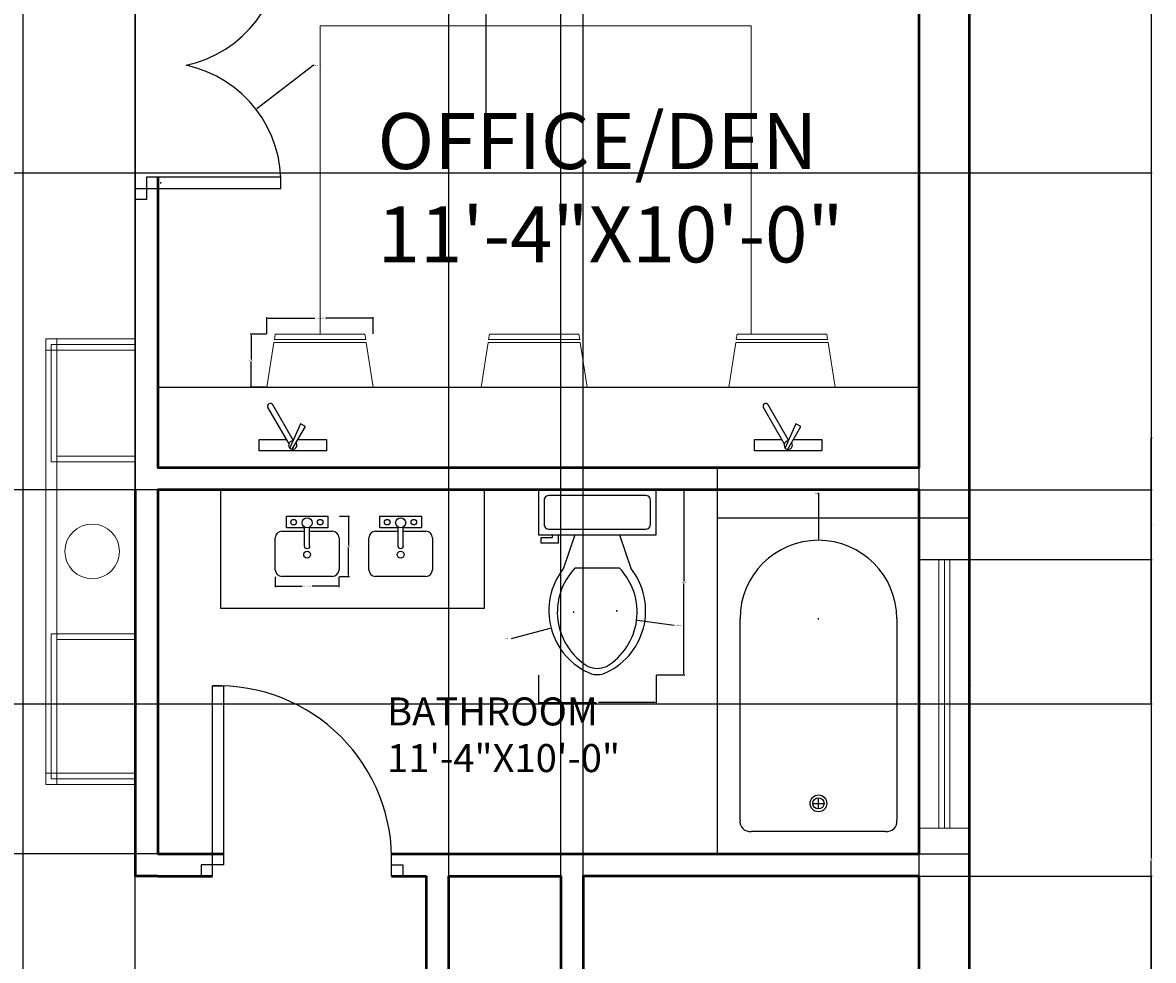
# Model space of a CAD drawing. Units: inches. Extents: x 821 to 2399, y 74 to 823.
# Tile 6 of 13: x 1128 to 1330, y 381 to 549. Entities that reach past the tile are written whole.
import ezdxf

# ---------------------------------------------------------------- set-up
doc = ezdxf.new("R2010")
doc.units = ezdxf.units.IN
doc.header["$MEASUREMENT"] = 0
doc.layers.get('0').update_dxf_attribs({"lineweight": 53})
for name, color, linetype, lineweight in [('A-ANNO-DIMS', 2, 'Continuous', 18), ('A-AREA-IDEN', 7, 'Continuous', 18), ('A-DOOR', 4, 'Continuous', 25), ('A-FLOR-CASE', 9, 'Continuous', 25), ('A-FLOR-FIXT', 8, 'Continuous', 25), ('A-FURN', 8, 'Continuous', 18), ('A-GLAZ', 4, 'Continuous', 18), ('WALLS', 7, 'Continuous', 50)]:
    doc.layers.add(name, color=color, linetype=linetype, lineweight=lineweight)
doc.styles.get("Standard").update_dxf_attribs({"font": 'arial.ttf'})
doc.dimstyles.get("Standard").update_dxf_attribs({"dimtxt": 0.18, "dimasz": 0.18, "dimexe": 0.18, "dimexo": 0.0625, "dimgap": 0.09, "dimtad": 0, "dimtih": 1, "dimtoh": 1, "dimdec": 4, "dimzin": 0, "dimdsep": 46, "dimtxsty": 'Standard', "dimcen": 0.09, "dimadec": 0, "dimazin": 0, "dimtfac": 1, "dimtdec": 4, "dimtofl": 0, "dimtmove": 0, "dimatfit": 3, "dimfxl": 1, "dimtolj": 1, "dimtzin": 0, "dimarcsym": 0})

# ---------------------------------------------------------------- blocks, each defined once
blk = doc.blocks.new('Bath Tub - 26 x 60 in.')
for p, q in [((8, -18), (10, -18)), ((9, -17), (9, -19))]:
    blk.add_line(p, q)
blk.add_lwpolyline([(0, -36), (0, 0), (60, 0), (60, -36)], close=True)
for points in [[(6, -4), (42, -4)], [(4, -30), (4, -6)], [(42, -32), (6, -32)]]:
    blk.add_lwpolyline(points)
for radius in [1.5, 1]:
    blk.add_circle((9, -18), radius)
for centre, radius, start, end in [((5.75, -5.75), 1.77, 81.8699, 188.1301), ((42, -18), 14, 270, 90), ((5.75, -30.25), 1.77, 171.8699, 278.1301)]:
    blk.add_arc(centre, radius, start, end)
blk = doc.blocks.new('Toilet - top')
for p, q in [((9.5, -6), (9.5, -2)), ((-8, -8.5), (-8, -8)), ((-7, -8), (-7, -9.5)), ((-4, -8), (-6, -14)), ((4, -8), (6, -14)), ((-10, -8.5), (-8, -8.5)), ((-10, -9.5), (-10, -8.5)), ((-7, -9.5), (-10, -9.5)), ((4, -14), (-4, -14))]:
    blk.add_line(p, q)
blk.add_lwpolyline([(10.5, -8), (10.5, 0), (-10.5, 0), (-10.5, -8)], close=True)
for points in [[(-9.5, -2), (-9.5, -6)], [(8.5, -1), (-8.5, -1)], [(-8.5, -7), (8.5, -7)]]:
    blk.add_lwpolyline(points)
for centre, radius, start, end in [((-8.62, -1.88), 0.884, 81.8699, 188.1301), ((8.62, -1.88), 0.884, 351.8699, 98.1301), ((-8.62, -6.12), 0.884, 171.8699, 278.1301), ((8.62, -6.12), 0.884, 261.8699, 8.1301), ((3.52, -21.58), 12.17, 141.4691, 247.9714), ((4.2, -21.82), 11.33, 136.3677, 238.9468), ((-3.52, -21.58), 12.17, 292.0284, 38.5307), ((-4.2, -21.82), 11.33, 301.053, 43.6321), ((0, -27.88), 4, 245.7318, 294.2682), ((0, -29), 4, 254.8605, 285.1395)]:
    blk.add_arc(centre, radius, start, end)
blk = doc.blocks.new('Faucet - single handle top')
for p, q in [((0.08, -0.26), (-2.26, -4.34)), ((-1.37, -4.79), (0.55, -0.5)), ((-0.06, -1.9), (3.57, -8.18)), ((4.43, -7.68), (0.72, -1.24)), ((-2.26, -4.34), (-1.37, -4.79))]:
    blk.add_line(p, q)
for points in [[(-0.92, -2), (-6, -2), (-6, 0), (6, 0), (6, -2), (1.16, -2)], [(-0.01, -2), (-0.12, -2)]]:
    blk.add_lwpolyline(points)
for centre, radius, start, end in [((0, -1), 0.75, 269.2246, 216.2304), ((4, -7.93), 0.5, 210, 30)]:
    blk.add_arc(centre, radius, start, end)
blk = doc.blocks.new('DOOR-SWING-32IN')
for p, q in [((0, 0), (2, 0)), ((34, 0), (36, 0))]:
    blk.add_line(p, q)
blk.add_lwpolyline([(34, 2, 0.433232), (2, 34), (4, 34), (4, 2), (2, 2), (2, 34)], format="xyb")
for points in [[(0, 0), (2, 0), (2, 2), (0, 2)], [(36, 0), (34, 0), (34, 2), (36, 2)]]:
    blk.add_lwpolyline(points, close=True)
blk = doc.blocks.new('WIN-48IN')
for p, q in [((3.5, 48), (3.5, 0)), ((4.5, 48), (4.5, 0)), ((5.5, 48), (5.5, 0))]:
    blk.add_line(p, q)
blk.add_lwpolyline([(9, 0), (0, 0), (0, 48), (9, 48)], close=True)
blk = doc.blocks.new('CHAIR-DESK-19IN')
for p, q in [((1.33, 8.5), (17.64, 8.5)), ((0, 0), (1.25, 8)), ((17.72, 8), (1.25, 8)), ((17.72, 8), (18.97, 0))]:
    blk.add_line(p, q)
blk.add_lwpolyline([(1.33, 8.5), (1.48, 9.5), (17.48, 9.5), (17.64, 8.5)])
blk = doc.blocks.new('LAV-RECT-WITH-FAUCET')
blk.add_line((6.15, 5.4), (6.15, 8.82))
for points in [[(5.25, 8.7), (2, 8.7), (2, 10.75), (5.8, 10.75)], [(5.8, 10.75), (9.4, 10.75), (9.4, 8.7), (6.15, 8.7)], [(1.2, 8.1), (5.25, 8.1)], [(6.15, 8.1), (10.2, 8.1)], [(0, 1.2), (0, 6.9)], [(11.4, 6.9), (11.4, 1.2)], [(10.2, 0), (1.2, 0)]]:
    blk.add_lwpolyline(points)
blk.add_lwpolyline([(6.15, 5.4, -1), (5.25, 5.4), (5.25, 8.82)], format="xyb")
for centre, radius in [((3.3, 9.7), 0.5), ((5.7, 9.6), 0.9), ((8.05, 9.7), 0.5), ((5.7, 3.9), 0.6)]:
    blk.add_circle(centre, radius)
for centre, start, end in [((1.28, 6.83), 93.3665, 176.6335), ((10.13, 6.83), 3.3665, 86.6335), ((1.28, 1.28), 183.3665, 266.6335), ((10.13, 1.28), 273.3665, 356.6335)]:
    blk.add_arc(centre, 1.28, start, end)
blk = doc.blocks.new('*D38')
at = {"layer": 'A-ANNO-DIMS', "color": 0, "lineweight": -2, "transparency": 16777216}
for p, q in [((1171.89, 493.43), (1171.89, 496.4)), ((1172.07, 496.22), (1180.42, 496.22)), ((1190.68, 496.22), (1182.32, 496.22)), ((1190.86, 493.43), (1190.86, 496.4))]:
    blk.add_line(p, q, dxfattribs=at)
at = {"layer": 'A-ANNO-DIMS', "color": 0, "lineweight": 50, "transparency": 16777216}
for points in [[(1172.07, 496.25), (1172.07, 496.19), (1171.89, 496.22)], [(1190.68, 496.25), (1190.68, 496.19), (1190.86, 496.22)]]:
    blk.add_solid(points, dxfattribs=at)
at = {"layer": 'Defpoints', "color": 0, "lineweight": 50, "transparency": 16777216}
for p in [(1190.86, 496.22), (1171.89, 493.37), (1190.86, 493.37)]:
    blk.add_point(p, dxfattribs=at)
at = {"layer": 'A-ANNO-DIMS', "color": 0, "transparency": 16777216, "insert": (1181.37, 496.22), "char_height": 0.18, "attachment_point": 5}
blk.add_mtext('\\A1;CHAIR 19 TYP.', dxfattribs=at)
blk = doc.blocks.new('*D39')
at = {"layer": 'A-ANNO-DIMS', "color": 0, "lineweight": -2, "transparency": 16777216}
for p, q in [((1171.82, 493.37), (1168.86, 493.37)), ((1169.04, 493.19), (1169.04, 488.8)), ((1169.04, 484.05), (1169.04, 488.44)), ((1171.82, 483.87), (1168.86, 483.87))]:
    blk.add_line(p, q, dxfattribs=at)
at = {"layer": 'A-ANNO-DIMS', "color": 0, "lineweight": 50, "transparency": 16777216}
for points in [[(1169.01, 493.19), (1169.07, 493.19), (1169.04, 493.37)], [(1169.01, 484.05), (1169.07, 484.05), (1169.04, 483.87)]]:
    blk.add_solid(points, dxfattribs=at)
at = {"layer": 'Defpoints', "color": 0, "lineweight": 50, "transparency": 16777216}
for p in [(1169.04, 493.37), (1171.89, 493.37), (1171.89, 483.87)]:
    blk.add_point(p, dxfattribs=at)
at = {"layer": 'A-ANNO-DIMS', "color": 0, "transparency": 16777216, "insert": (1169.04, 488.62), "char_height": 0.18, "attachment_point": 5}
blk.add_mtext('\\A1;10 TYP.', dxfattribs=at)
blk = doc.blocks.new('*D42')
at = {"layer": 'A-ANNO-DIMS', "color": 0, "lineweight": -2, "transparency": 16777216}
for p, q in [((1173.35, 450), (1173.35, 448.17)), ((1173.53, 448.35), (1178.12, 448.35)), ((1184.57, 448.35), (1179.99, 448.35)), ((1184.75, 450), (1184.75, 448.17))]:
    blk.add_line(p, q, dxfattribs=at)
at = {"layer": 'A-ANNO-DIMS', "color": 0, "lineweight": 50, "transparency": 16777216}
for points in [[(1173.53, 448.38), (1173.53, 448.32), (1173.35, 448.35)], [(1184.57, 448.38), (1184.57, 448.32), (1184.75, 448.35)]]:
    blk.add_solid(points, dxfattribs=at)
at = {"layer": 'Defpoints', "color": 0, "lineweight": 50, "transparency": 16777216}
for p in [(1173.35, 450.06), (1184.75, 450.06), (1184.75, 448.35)]:
    blk.add_point(p, dxfattribs=at)
at = {"layer": 'A-ANNO-DIMS', "color": 0, "transparency": 16777216, "insert": (1179.05, 448.35), "char_height": 0.18, "attachment_point": 5}
blk.add_mtext('\\A1;BASIN 11 TYP.', dxfattribs=at)
blk = doc.blocks.new('*D43')
at = {"layer": 'A-ANNO-DIMS', "color": 0, "lineweight": -2, "transparency": 16777216}
for p, q in [((1184.82, 460.81), (1186.64, 460.81)), ((1186.46, 460.63), (1186.46, 455.61)), ((1186.46, 450.24), (1186.46, 455.25)), ((1184.82, 450.06), (1186.64, 450.06))]:
    blk.add_line(p, q, dxfattribs=at)
at = {"layer": 'A-ANNO-DIMS', "color": 0, "lineweight": 50, "transparency": 16777216}
for points in [[(1186.43, 460.63), (1186.49, 460.63), (1186.46, 460.81)], [(1186.43, 450.24), (1186.49, 450.24), (1186.46, 450.06)]]:
    blk.add_solid(points, dxfattribs=at)
at = {"layer": 'Defpoints', "color": 0, "lineweight": 50, "transparency": 16777216}
for p in [(1184.75, 460.81), (1186.46, 460.81), (1184.75, 450.06)]:
    blk.add_point(p, dxfattribs=at)
at = {"layer": 'A-ANNO-DIMS', "color": 0, "transparency": 16777216, "insert": (1186.46, 455.43), "char_height": 0.18, "attachment_point": 5}
blk.add_mtext('\\A1;11 TYP.', dxfattribs=at)
blk = doc.blocks.new('*D54')
at = {"layer": 'A-ANNO-DIMS', "color": 0, "lineweight": -2, "transparency": 16777216}
for p, q in [((1288.44, 460.52), (1297.55, 460.52)), ((1297.37, 460.34), (1297.37, 430.7)), ((1297.37, 400.7), (1297.37, 430.34)), ((1288.44, 400.52), (1297.55, 400.52))]:
    blk.add_line(p, q, dxfattribs=at)
at = {"layer": 'A-ANNO-DIMS', "color": 0, "lineweight": 50, "transparency": 16777216}
for points in [[(1297.34, 460.34), (1297.4, 460.34), (1297.37, 460.52)], [(1297.34, 400.7), (1297.4, 400.7), (1297.37, 400.52)]]:
    blk.add_solid(points, dxfattribs=at)
at = {"layer": 'Defpoints', "color": 0, "lineweight": 50, "transparency": 16777216}
for p in [(1288.37, 460.52), (1297.37, 460.52), (1288.37, 400.52)]:
    blk.add_point(p, dxfattribs=at)
at = {"layer": 'A-ANNO-DIMS', "color": 0, "transparency": 16777216, "insert": (1297.37, 430.52), "char_height": 0.18, "attachment_point": 5}
blk.add_mtext('\\A1;TUB 60', dxfattribs=at)
blk = doc.blocks.new('*D55')
at = {"layer": 'A-ANNO-DIMS', "color": 0, "lineweight": -2, "transparency": 16777216}
for p, q in [((1252.37, 460.58), (1252.37, 469.7)), ((1252.55, 469.52), (1270.15, 469.52)), ((1288.19, 469.52), (1270.59, 469.52)), ((1288.37, 460.58), (1288.37, 469.7))]:
    blk.add_line(p, q, dxfattribs=at)
at = {"layer": 'A-ANNO-DIMS', "color": 0, "lineweight": 50, "transparency": 16777216}
for points in [[(1252.55, 469.55), (1252.55, 469.49), (1252.37, 469.52)], [(1288.19, 469.55), (1288.19, 469.49), (1288.37, 469.52)]]:
    blk.add_solid(points, dxfattribs=at)
at = {"layer": 'Defpoints', "color": 0, "lineweight": 50, "transparency": 16777216}
for p in [(1252.37, 469.52), (1252.37, 460.52), (1288.37, 460.52)]:
    blk.add_point(p, dxfattribs=at)
at = {"layer": 'A-ANNO-DIMS', "color": 0, "transparency": 16777216, "insert": (1270.37, 469.52), "char_height": 0.18, "attachment_point": 5}
blk.add_mtext('\\A1;36', dxfattribs=at)
blk = doc.blocks.new('*D56')
at = {"layer": 'A-ANNO-DIMS', "color": 0, "lineweight": -2, "transparency": 16777216}
for p, q in [((1241.44, 465.52), (1246.51, 465.52)), ((1246.33, 465.34), (1246.33, 449.18)), ((1246.33, 432.65), (1246.33, 448.81)), ((1241.44, 432.47), (1246.51, 432.47))]:
    blk.add_line(p, q, dxfattribs=at)
at = {"layer": 'A-ANNO-DIMS', "color": 0, "lineweight": 50, "transparency": 16777216}
for points in [[(1246.3, 465.34), (1246.36, 465.34), (1246.33, 465.52)], [(1246.3, 432.65), (1246.36, 432.65), (1246.33, 432.47)]]:
    blk.add_solid(points, dxfattribs=at)
at = {"layer": 'Defpoints', "color": 0, "lineweight": 50, "transparency": 16777216}
for p in [(1241.37, 465.52), (1246.33, 465.52), (1241.37, 432.47)]:
    blk.add_point(p, dxfattribs=at)
at = {"layer": 'A-ANNO-DIMS', "color": 0, "transparency": 16777216, "insert": (1246.33, 449), "char_height": 0.18, "attachment_point": 5}
blk.add_mtext('\\A1;WC 33', dxfattribs=at)
blk = doc.blocks.new('*D57')
at = {"layer": 'A-ANNO-DIMS', "color": 0, "lineweight": -2, "transparency": 16777216}
for p, q in [((1220.37, 432.41), (1220.37, 427.34)), ((1241.37, 432.41), (1241.37, 427.34)), ((1220.55, 427.52), (1230.67, 427.52)), ((1241.19, 427.52), (1231.08, 427.52))]:
    blk.add_line(p, q, dxfattribs=at)
at = {"layer": 'A-ANNO-DIMS', "color": 0, "lineweight": 50, "transparency": 16777216}
for points in [[(1220.55, 427.55), (1220.55, 427.49), (1220.37, 427.52)], [(1241.19, 427.55), (1241.19, 427.49), (1241.37, 427.52)]]:
    blk.add_solid(points, dxfattribs=at)
at = {"layer": 'Defpoints', "color": 0, "lineweight": 50, "transparency": 16777216}
for p in [(1220.37, 432.47), (1241.37, 432.47), (1241.37, 427.52)]:
    blk.add_point(p, dxfattribs=at)
at = {"layer": 'A-ANNO-DIMS', "color": 0, "transparency": 16777216, "insert": (1230.87, 427.52), "char_height": 0.18, "attachment_point": 5}
blk.add_mtext('\\A1;21', dxfattribs=at)
blk = doc.blocks.new('*D79')
at = {"layer": 'A-ANNO-DIMS', "color": 0, "lineweight": -2, "transparency": 16777216}
for p, q in [((1297.44, 598.52), (1330, 598.52)), ((1329.82, 598.34), (1329.82, 399.7)), ((1329.82, 200.7), (1329.82, 399.34)), ((1297.44, 200.52), (1330, 200.52))]:
    blk.add_line(p, q, dxfattribs=at)
at = {"layer": 'A-ANNO-DIMS', "color": 0, "lineweight": 50, "transparency": 16777216}
for points in [[(1329.79, 598.34), (1329.85, 598.34), (1329.82, 598.52)], [(1329.79, 200.7), (1329.85, 200.7), (1329.82, 200.52)]]:
    blk.add_solid(points, dxfattribs=at)
at = {"layer": 'Defpoints', "color": 0, "lineweight": 50, "transparency": 16777216}
for p in [(1297.37, 598.52), (1297.37, 200.52), (1329.82, 200.52)]:
    blk.add_point(p, dxfattribs=at)
at = {"layer": 'A-ANNO-DIMS', "color": 0, "transparency": 16777216, "insert": (1329.82, 399.52), "char_height": 0.18, "attachment_point": 5}
blk.add_mtext('\\A1;398', dxfattribs=at)
blk = doc.blocks.new('*D92')
at = {"layer": 'A-ANNO-DIMS', "color": 0, "lineweight": -2, "transparency": 16777216}
for p, q in [((1128.37, 209.58), (1128.37, 786.75)), ((1128.55, 786.57), (1138.15, 786.57)), ((1148.19, 786.57), (1138.59, 786.57)), ((1148.37, 209.58), (1148.37, 786.75))]:
    blk.add_line(p, q, dxfattribs=at)
at = {"layer": 'A-ANNO-DIMS', "color": 0, "lineweight": 50, "transparency": 16777216}
for points in [[(1128.55, 786.6), (1128.55, 786.54), (1128.37, 786.57)], [(1148.19, 786.6), (1148.19, 786.54), (1148.37, 786.57)]]:
    blk.add_solid(points, dxfattribs=at)
at = {"layer": 'Defpoints', "color": 0, "lineweight": 50, "transparency": 16777216}
for p in [(1148.37, 786.57), (1128.37, 209.52), (1148.37, 209.52)]:
    blk.add_point(p, dxfattribs=at)
at = {"layer": 'A-ANNO-DIMS', "color": 0, "transparency": 16777216, "insert": (1138.37, 786.57), "char_height": 0.18, "attachment_point": 5}
blk.add_mtext('\\A1;20', dxfattribs=at)
blk = doc.blocks.new('*D94')
at = {"layer": 'A-ANNO-DIMS', "color": 0, "lineweight": -2, "transparency": 16777216}
for p, q in [((1204.37, 396.58), (1204.37, 786.75)), ((1204.55, 786.57), (1214.15, 786.57)), ((1224.19, 786.57), (1214.59, 786.57)), ((1224.37, 396.58), (1224.37, 786.75))]:
    blk.add_line(p, q, dxfattribs=at)
at = {"layer": 'A-ANNO-DIMS', "color": 0, "lineweight": 50, "transparency": 16777216}
for points in [[(1204.55, 786.6), (1204.55, 786.54), (1204.37, 786.57)], [(1224.19, 786.6), (1224.19, 786.54), (1224.37, 786.57)]]:
    blk.add_solid(points, dxfattribs=at)
at = {"layer": 'Defpoints', "color": 0, "lineweight": 50, "transparency": 16777216}
for p in [(1224.37, 786.57), (1204.37, 396.52), (1224.37, 396.52)]:
    blk.add_point(p, dxfattribs=at)
at = {"layer": 'A-ANNO-DIMS', "color": 0, "transparency": 16777216, "insert": (1214.37, 786.57), "char_height": 0.18, "attachment_point": 5}
blk.add_mtext('\\A1;20', dxfattribs=at)
blk = doc.blocks.new('*D95')
at = {"layer": 'A-ANNO-DIMS', "color": 0, "lineweight": -2, "transparency": 16777216}
for p, q in [((1228.37, 396.58), (1228.37, 786.75)), ((1228.55, 786.57), (1258.15, 786.57)), ((1288.19, 786.57), (1258.59, 786.57)), ((1288.37, 396.58), (1288.37, 786.75))]:
    blk.add_line(p, q, dxfattribs=at)
at = {"layer": 'A-ANNO-DIMS', "color": 0, "lineweight": 50, "transparency": 16777216}
for points in [[(1228.55, 786.6), (1228.55, 786.54), (1228.37, 786.57)], [(1288.19, 786.6), (1288.19, 786.54), (1288.37, 786.57)]]:
    blk.add_solid(points, dxfattribs=at)
at = {"layer": 'Defpoints', "color": 0, "lineweight": 50, "transparency": 16777216}
for p in [(1288.37, 786.57), (1228.37, 396.52), (1288.37, 396.52)]:
    blk.add_point(p, dxfattribs=at)
at = {"layer": 'A-ANNO-DIMS', "color": 0, "transparency": 16777216, "insert": (1258.37, 786.57), "char_height": 0.18, "attachment_point": 5}
blk.add_mtext('\\A1;60', dxfattribs=at)
blk = doc.blocks.new('*D96')
at = {"layer": 'A-ANNO-DIMS', "color": 0, "lineweight": -2, "transparency": 16777216}
for p, q in [((1288.44, 396.52), (1330, 396.52)), ((1329.82, 396.34), (1329.82, 371.2)), ((1329.82, 345.7), (1329.82, 370.84)), ((1288.44, 345.52), (1330, 345.52))]:
    blk.add_line(p, q, dxfattribs=at)
at = {"layer": 'A-ANNO-DIMS', "color": 0, "lineweight": 50, "transparency": 16777216}
for points in [[(1329.79, 396.34), (1329.85, 396.34), (1329.82, 396.52)], [(1329.79, 345.7), (1329.85, 345.7), (1329.82, 345.52)]]:
    blk.add_solid(points, dxfattribs=at)
at = {"layer": 'Defpoints', "color": 0, "lineweight": 50, "transparency": 16777216}
for p in [(1288.37, 396.52), (1288.37, 345.52), (1329.82, 345.52)]:
    blk.add_point(p, dxfattribs=at)
at = {"layer": 'A-ANNO-DIMS', "color": 0, "transparency": 16777216, "insert": (1329.82, 371.02), "char_height": 0.18, "attachment_point": 5}
blk.add_mtext('\\A1;51', dxfattribs=at)
blk = doc.blocks.new('*D97')
at = {"layer": 'A-ANNO-DIMS', "color": 0, "lineweight": -2, "transparency": 16777216}
for p, q in [((1152.31, 465.52), (820.74, 465.52)), ((820.92, 465.34), (820.92, 433.2)), ((820.92, 400.7), (820.92, 432.84)), ((1152.31, 400.52), (820.74, 400.52))]:
    blk.add_line(p, q, dxfattribs=at)
at = {"layer": 'A-ANNO-DIMS', "color": 0, "lineweight": 50, "transparency": 16777216}
for points in [[(820.89, 465.34), (820.95, 465.34), (820.92, 465.52)], [(820.89, 400.7), (820.95, 400.7), (820.92, 400.52)]]:
    blk.add_solid(points, dxfattribs=at)
at = {"layer": 'Defpoints', "color": 0, "lineweight": 50, "transparency": 16777216}
for p in [(820.92, 465.52), (1152.37, 465.52), (1152.37, 400.52)]:
    blk.add_point(p, dxfattribs=at)
at = {"layer": 'A-ANNO-DIMS', "color": 0, "transparency": 16777216, "insert": (820.92, 433.02), "char_height": 0.18, "attachment_point": 5}
blk.add_mtext('\\A1;65', dxfattribs=at)
blk = doc.blocks.new('*D99')
at = {"layer": 'A-ANNO-DIMS', "color": 0, "lineweight": -2, "transparency": 16777216}
for p, q in [((1288.44, 465.52), (1330, 465.52)), ((1329.82, 465.34), (1329.82, 459.48)), ((1329.82, 453.25), (1329.82, 459.11)), ((1288.44, 453.07), (1330, 453.07))]:
    blk.add_line(p, q, dxfattribs=at)
at = {"layer": 'A-ANNO-DIMS', "color": 0, "lineweight": 50, "transparency": 16777216}
for points in [[(1329.79, 465.34), (1329.85, 465.34), (1329.82, 465.52)], [(1329.79, 453.25), (1329.85, 453.25), (1329.82, 453.07)]]:
    blk.add_solid(points, dxfattribs=at)
at = {"layer": 'Defpoints', "color": 0, "lineweight": 50, "transparency": 16777216}
for p in [(1288.37, 465.52), (1288.37, 453.07), (1329.82, 453.07)]:
    blk.add_point(p, dxfattribs=at)
at = {"layer": 'A-ANNO-DIMS', "color": 0, "transparency": 16777216, "insert": (1329.82, 459.29), "char_height": 0.18, "attachment_point": 5}
blk.add_mtext('\\A1;12.452', dxfattribs=at)
blk = doc.blocks.new('*D103')
at = {"layer": 'A-ANNO-DIMS', "color": 0, "lineweight": -2, "transparency": 16777216}
for p, q in [((966.67, 522.18), (1330, 522.18)), ((1329.82, 522), (1329.82, 474.94)), ((1329.82, 427.51), (1329.82, 474.57)), ((966.67, 427.33), (1330, 427.33))]:
    blk.add_line(p, q, dxfattribs=at)
at = {"layer": 'A-ANNO-DIMS', "color": 0, "lineweight": 50, "transparency": 16777216}
for points in [[(1329.79, 522), (1329.85, 522), (1329.82, 522.18)], [(1329.79, 427.51), (1329.85, 427.51), (1329.82, 427.33)]]:
    blk.add_solid(points, dxfattribs=at)
at = {"layer": 'Defpoints', "color": 0, "lineweight": 50, "transparency": 16777216}
for p in [(966.61, 522.18), (1329.82, 522.18), (966.61, 427.33)]:
    blk.add_point(p, dxfattribs=at)
at = {"layer": 'A-ANNO-DIMS', "color": 0, "transparency": 16777216, "insert": (1329.82, 474.75), "char_height": 0.18, "attachment_point": 5}
blk.add_mtext('\\A1;94.85', dxfattribs=at)
blk = doc.blocks.new('*D138')
at = {"layer": 'A-ANNO-DIMS', "color": 0, "lineweight": -2, "transparency": 16777216}
for p, q in [((1210.94, 629.52), (1211.12, 629.52)), ((1211.03, 629.43), (1211.03, 629.61)), ((1211.03, 531.92), (1211.03, 568.34)), ((1211.21, 531.92), (1211.03, 531.92))]:
    blk.add_line(p, q, dxfattribs=at)
at = {"layer": 'A-ANNO-DIMS', "color": 0, "lineweight": 50, "transparency": 16777216}
blk.add_solid([(1211.06, 568.34), (1211, 568.34), (1211.03, 568.52)], dxfattribs=at)
at = {"layer": 'Defpoints', "color": 0, "lineweight": 50, "transparency": 16777216}
for p in [(1211.03, 629.52), (1211.03, 568.52)]:
    blk.add_point(p, dxfattribs=at)
at = {"layer": 'A-ANNO-DIMS', "color": 0, "transparency": 16777216, "insert": (1211.5, 531.92), "char_height": 0.18, "attachment_point": 5}
blk.add_mtext('\\A1;R61', dxfattribs=at)
blk = doc.blocks.new('*D139')
at = {"layer": 'A-ANNO-DIMS', "color": 0, "lineweight": -2, "transparency": 16777216}
for p, q in [((1270.19, 464.92), (1270.37, 464.92)), ((1270.37, 464.92), (1270.37, 456.7)), ((1270.28, 442.52), (1270.46, 442.52)), ((1270.37, 442.43), (1270.37, 442.61))]:
    blk.add_line(p, q, dxfattribs=at)
at = {"layer": 'A-ANNO-DIMS', "color": 0, "lineweight": 50, "transparency": 16777216}
blk.add_solid([(1270.4, 456.7), (1270.34, 456.7), (1270.37, 456.52)], dxfattribs=at)
at = {"layer": 'Defpoints', "color": 0, "lineweight": 50, "transparency": 16777216}
for p in [(1270.37, 456.52), (1270.37, 442.52)]:
    blk.add_point(p, dxfattribs=at)
at = {"layer": 'A-ANNO-DIMS', "color": 0, "transparency": 16777216, "insert": (1269.89, 464.92), "char_height": 0.18, "attachment_point": 5}
blk.add_mtext('\\A1;R14', dxfattribs=at)
blk = doc.blocks.new('*D140')
at = {"layer": 'A-ANNO-DIMS', "color": 0, "lineweight": -2, "transparency": 16777216}
for p, q in [((1234.3, 443.94), (1234.48, 443.94)), ((1234.39, 443.85), (1234.39, 444.03)), ((1215.56, 438.99), (1222.45, 440.8))]:
    blk.add_line(p, q, dxfattribs=at)
at = {"layer": 'A-ANNO-DIMS', "color": 0, "lineweight": 50, "transparency": 16777216}
blk.add_solid([(1222.44, 440.83), (1222.46, 440.77), (1222.62, 440.85)], dxfattribs=at)
at = {"layer": 'Defpoints', "color": 0, "lineweight": 50, "transparency": 16777216}
for p in [(1234.39, 443.94), (1222.62, 440.85)]:
    blk.add_point(p, dxfattribs=at)
at = {"layer": 'A-ANNO-DIMS', "color": 0, "transparency": 16777216, "insert": (1214.89, 438.99), "char_height": 0.18, "attachment_point": 5}
blk.add_mtext('\\A1;2X R12.17', dxfattribs=at)
blk = doc.blocks.new('*D141')
at = {"layer": 'A-ANNO-DIMS', "color": 0, "lineweight": -2, "transparency": 16777216}
for p, q in [((1226.58, 443.7), (1226.76, 443.7)), ((1226.67, 443.61), (1226.67, 443.79)), ((1244.64, 441.29), (1238.08, 442.17))]:
    blk.add_line(p, q, dxfattribs=at)
at = {"layer": 'A-ANNO-DIMS', "color": 0, "lineweight": 50, "transparency": 16777216}
blk.add_solid([(1238.08, 442.2), (1238.08, 442.14), (1237.9, 442.19)], dxfattribs=at)
at = {"layer": 'Defpoints', "color": 0, "lineweight": 50, "transparency": 16777216}
for p in [(1226.67, 443.7), (1237.9, 442.19)]:
    blk.add_point(p, dxfattribs=at)
at = {"layer": 'A-ANNO-DIMS', "color": 0, "transparency": 16777216, "insert": (1245.31, 441.29), "char_height": 0.18, "attachment_point": 5}
blk.add_mtext('\\A1;2X R11.33', dxfattribs=at)
blk = doc.blocks.new('*D142')
at = {"layer": 'A-ANNO-DIMS', "color": 0, "lineweight": -2, "transparency": 16777216}
for p, q in [((1180.16, 541.35), (1170.08, 533.6)), ((1180.34, 541.35), (1180.16, 541.35)), ((1152.82, 520.39), (1153, 520.39)), ((1152.91, 520.3), (1152.91, 520.48))]:
    blk.add_line(p, q, dxfattribs=at)
at = {"layer": 'A-ANNO-DIMS', "color": 0, "lineweight": 50, "transparency": 16777216}
blk.add_solid([(1170.07, 533.63), (1170.1, 533.58), (1169.94, 533.49)], dxfattribs=at)
at = {"layer": 'Defpoints', "color": 0, "lineweight": 50, "transparency": 16777216}
for p in [(1169.94, 533.49), (1152.91, 520.39)]:
    blk.add_point(p, dxfattribs=at)
at = {"layer": 'A-ANNO-DIMS', "color": 0, "transparency": 16777216, "insert": (1181.09, 541.35), "char_height": 0.18, "attachment_point": 5}
blk.add_mtext('\\A1;4X R21.485', dxfattribs=at)

msp = doc.modelspace()

# ---------------------------------------------------------------- linework, layer by layer
at = {"layer": 'A-DOOR'}
msp.add_lwpolyline([(1174.3735, 519.3933), (1174.3735, 521.3933), (1150.3735, 521.3933), (1150.3735, 519.3933), (1174.3735, 519.3933, 0.36630785), (1157.4504, 541.3933, 0.36630785), (1174.3735, 563.3933), (1174.3735, 561.3933), (1150.3735, 561.3933), (1150.3735, 563.3933), (1148.3735, 563.3933), (1148.3735, 519.3933), (1150.3735, 519.3933), (1150.3735, 517.3933), (1148.3735, 517.3933), (1148.3735, 519.3933), (1148.3735, 465.5195)], format="xyb", dxfattribs=at)
at = {"layer": 'A-FLOR-CASE'}
msp.add_line((1152.3735, 483.8678), (1288.3735, 483.8678), dxfattribs=at)
msp.add_lwpolyline([(1163.6073, 465.5195), (1163.6073, 444.3825), (1210.7669, 444.3825), (1210.7669, 465.5195)], dxfattribs=at)
at = {"layer": 'A-FURN'}
for p, q in [((1134.3735, 412.9198), (1134.3735, 492.5195)), ((1132.3735, 490.5195), (1148.3735, 490.5195)), ((1132.3735, 414.9198), (1148.3735, 414.9198))]:
    msp.add_line(p, q, dxfattribs=at)
for points in [[(1181.3708, 493.3702), (1181.3708, 548.4276), (1258.3361, 548.4276), (1258.3361, 493.3702)], [(1148.3735, 412.9198), (1132.3735, 412.9198), (1132.3735, 492.5195), (1148.3735, 492.5195)], [(1148.3735, 470.5494), (1133.3735, 470.5494), (1133.3735, 491.5195), (1148.3735, 491.5195)], [(1148.3735, 413.9198), (1133.3735, 413.9198), (1133.3735, 439.7905), (1148.3735, 439.7905)]]:
    msp.add_lwpolyline(points, dxfattribs=at)
for points in [[(1134.3735, 490.5195), (1148.3735, 490.5195), (1148.3735, 471.5494), (1134.3735, 471.5494)], [(1134.3735, 438.7905), (1148.3735, 438.7905), (1148.3735, 414.9198), (1134.3735, 414.9198)]]:
    msp.add_lwpolyline(points, close=True, dxfattribs=at)
msp.add_circle((1140.6752, 454.5503), 4.8838, dxfattribs=at)
at = {"layer": 'WALLS'}
for p, q in [((1148.3735, 465.5195), (1148.3735, 396.5195)), ((1152.3735, 396.5195), (1148.3735, 396.5195)), ((1152.3735, 396.5195), (1162.139, 396.5195)), ((1194.139, 396.5195), (1200.3735, 396.5195)), ((1200.3735, 345.5195), (1200.3735, 396.5195))]:
    msp.add_line(p, q, dxfattribs=at)
for points in [[(1050.641, 200.5195), (1050.641, 170.9407), (1121.9086, 170.9407), (1128.124, 170.9407), (1050.641, 170.9407), (1050.641, 106.8645), (1128.124, 106.8645), (1128.124, 170.9407), (1128.124, 200.5195), (1288.3735, 200.5195), (1297.3735, 200.5195), (1297.3735, 598.5195), (853.3735, 598.5195), (853.3735, 292.549), (922.3673, 292.5195), (1043.3735, 292.5195), (1043.3735, 209.5195), (1043.3735, 200.5195)], [(1204.3735, 345.5195), (1204.3735, 396.5195), (1224.3735, 396.5195), (1224.3735, 345.5195)], [(1288.3735, 396.5195), (1228.3735, 396.5195), (1228.3735, 345.5195), (1288.3735, 345.5195)]]:
    msp.add_lwpolyline(points, close=True, dxfattribs=at)
for points in [[(1152.3735, 521.3933), (1152.3735, 469.5195), (1288.3735, 469.5195), (1288.3735, 589.5195), (1152.3735, 589.5195), (1152.3735, 561.3933)], [(1194.139, 400.5195), (1288.3735, 400.5195), (1288.3735, 465.5195), (1152.3735, 465.5195), (1152.3735, 400.5195), (1164.139, 400.5195)]]:
    msp.add_lwpolyline(points, dxfattribs=at)

# ---------------------------------------------------------------- block references
at = {"layer": 'A-DOOR'}
msp.add_blockref('DOOR-SWING-32IN', (1160.1385, 396.519), dxfattribs=at)
at = {"layer": 'A-FLOR-FIXT'}
for name, p, rotation in [('Faucet - single handle top', (1176.4954, 472.5259), 180), ('Faucet - single handle top', (1264.9849, 472.5259), 180), ('Bath Tub - 26 x 60 in.', (1252.3735, 400.5195), 90)]:
    msp.add_blockref(name, p, dxfattribs=dict(at, rotation=rotation))
for name, p in [('Toilet - top', (1230.8735, 465.5195)), ('LAV-RECT-WITH-FAUCET', (1173.3534, 450.058)), ('LAV-RECT-WITH-FAUCET', (1190.067, 450.058))]:
    msp.add_blockref(name, p, dxfattribs=at)
at = {"layer": 'A-FURN'}
for p in [(1171.886, 483.868), (1210.1321, 483.868), (1254.382, 483.868)]:
    msp.add_blockref('CHAIR-DESK-19IN', p, dxfattribs=at)
at = {"layer": 'A-GLAZ'}
msp.add_blockref('WIN-48IN', (1288.373, 405.067), dxfattribs=at)

# ---------------------------------------------------------------- texts
at = {"layer": 'A-AREA-IDEN', "attachment_point": 1}
for s, width, insert, char_height in [('OFFICE/DEN\\P11\'-4"X10\'-0"', 56.022718, (1191.6348, 532.8458), 10), ('BATHROOM\\P11\'-4"X10\'-0"', 59.045639, (1193.3278, 428.4482), 5)]:
    msp.add_mtext_dynamic_manual_height_columns(s, width=width, gutter_width=1, heights=[0], dxfattribs=dict(at, insert=insert, char_height=char_height))

# ---------------------------------------------------------------- dimensions: what is measured, and where the dimension line sits
at = {"layer": 'A-ANNO-DIMS'}
for base, p1, p2, picture, middle in [((1148.3735, 786.5664), (1128.3735, 209.5195), (1148.3735, 209.5195), '*D92', (1138.3735, 786.5664)), ((1224.3735, 786.5664), (1204.3735, 396.5195), (1224.3735, 396.5195), '*D94', (1214.3735, 786.5664)), ((1288.3735, 786.5664), (1228.3735, 396.5195), (1288.3735, 396.5195), '*D95', (1258.3735, 786.5664)), ((1241.3735, 427.5163), (1220.3735, 432.4732), (1241.3735, 432.4732), '*D57', (1230.8735, 427.5163))]:
    dim = msp.add_linear_dim(base=base, p1=p1, p2=p2, dimstyle='Standard', override={"dimdec": 0, "dimlfac": 1, "dimrnd": 0, "dimzin": 0, "dimdsep": 46, "dimlunit": 2}, dxfattribs=at)
    dim.commit()
    dim.dimension.update_dxf_attribs({"geometry": picture, "text_midpoint": middle})
for center, mpoint, picture, middle in [((1211.0276, 629.5195), (1211.028, 568.5195), '*D138', (1211.4959, 531.9195)), ((1270.3735, 442.5195), (1270.373, 456.5195), '*D139', (1269.888, 464.9195))]:
    dim = msp.add_radius_dim(center=center, mpoint=mpoint, dimstyle='Standard', override={"dimdec": 0, "dimlfac": 1, "dimrnd": 0, "dimzin": 0, "dimdsep": 46, "dimlunit": 2}, dxfattribs=at)
    dim.commit()
    dim.dimension.update_dxf_attribs({"geometry": picture, "text_midpoint": middle, "dimtype": 164})
for base, p1, p2, angle, override, picture, middle in [((1329.8235, 200.5195), (1297.3735, 598.5195), (1297.3735, 200.5195), 90, {"dimdec": 0, "dimlfac": 1, "dimrnd": 0, "dimzin": 0, "dimdsep": 46, "dimlunit": 2}, '*D79', (1329.8235, 399.5195)), ((1329.8235, 522.1769), (966.6107, 427.3294), (966.6107, 522.1769), 90, {"dimdec": 2, "dimlfac": 1, "dimrnd": 0, "dimzin": 0, "dimdsep": 46, "dimlunit": 2}, '*D103', (1329.8235, 474.7531)), ((1252.3735, 469.5195), (1288.3735, 460.5195), (1252.3735, 460.5195), 180, {"dimdec": 0, "dimlfac": 1, "dimrnd": 0, "dimzin": 0, "dimdsep": 46, "dimlunit": 2}, '*D55', (1270.3735, 469.5195)), ((820.9235, 465.5195), (1152.3735, 400.5195), (1152.3735, 465.5195), 90, {"dimdec": 0, "dimlfac": 1, "dimrnd": 0, "dimzin": 0, "dimdsep": 46, "dimlunit": 2}, '*D97', (820.9235, 433.0195)), ((1329.8235, 453.0671), (1288.3735, 465.5195), (1288.3735, 453.0671), 90, {"dimdec": 3, "dimlfac": 1, "dimrnd": 0, "dimzin": 0, "dimdsep": 46, "dimlunit": 2}, '*D99', (1329.8235, 459.2933)), ((1329.8235, 345.5195), (1288.3735, 396.5195), (1288.3735, 345.5195), 90, {"dimdec": 0, "dimlfac": 1, "dimrnd": 0, "dimzin": 0, "dimdsep": 46, "dimlunit": 2}, '*D96', (1329.8235, 371.0195))]:
    dim = msp.add_linear_dim(base=base, p1=p1, p2=p2, angle=angle, dimstyle='Standard', override=override, dxfattribs=at)
    dim.commit()
    dim.dimension.update_dxf_attribs({"geometry": picture, "text_midpoint": middle})
for center, mpoint, text, override, picture, middle in [((1152.9119, 520.3933), (1169.9411, 533.4931), '4X <>', {"dimdec": 3, "dimlfac": 1, "dimrnd": 0, "dimzin": 0, "dimdsep": 46, "dimlunit": 2}, '*D142', (1181.0861, 541.353)), ((1234.393, 443.939), (1222.6233, 440.8471), '2X <>', {"dimdec": 2, "dimlfac": 1, "dimrnd": 0, "dimzin": 0, "dimdsep": 46, "dimlunit": 2}, '*D140', (1215.5615, 438.992)), ((1226.6736, 443.7021), (1237.9017, 442.192), '2X <>', {"dimdec": 2, "dimlfac": 1, "dimrnd": 0, "dimzin": 0, "dimdsep": 46, "dimlunit": 2}, '*D141', (1244.6385, 441.286))]:
    dim = msp.add_radius_dim(center=center, mpoint=mpoint, text=text, dimstyle='Standard', override=override, dxfattribs=at)
    dim.commit()
    dim.dimension.update_dxf_attribs({"geometry": picture, "text_midpoint": middle, "dimtype": 164})
for base, p1, p2, text, picture, middle in [((1190.8555, 496.2156), (1171.886, 493.3702), (1190.8555, 493.3702), 'CHAIR <> TYP.', '*D38', (1181.3708, 496.2156)), ((1184.7537, 448.3482), (1173.3536, 450.0582), (1184.7537, 450.0582), 'BASIN <> TYP.', '*D42', (1179.0536, 448.3482))]:
    dim = msp.add_linear_dim(base=base, p1=p1, p2=p2, text=text, dimstyle='Standard', override={"dimdec": 0, "dimlfac": 1, "dimrnd": 0, "dimzin": 0, "dimdsep": 46, "dimlunit": 2}, dxfattribs=at)
    dim.commit()
    dim.dimension.update_dxf_attribs({"geometry": picture, "text_midpoint": middle})
for base, p1, p2, text, picture, middle in [((1169.0406, 493.3702), (1171.886, 483.8678), (1171.886, 493.3702), '<> TYP.', '*D39', (1169.0406, 488.619)), ((1246.3304, 465.5195), (1241.3735, 432.4732), (1241.3735, 465.5195), 'WC <>', '*D56', (1246.3304, 448.9963)), ((1186.4637, 460.8082), (1184.7537, 450.0582), (1184.7537, 460.8082), '<> TYP.', '*D43', (1186.4637, 455.4332)), ((1297.3735, 460.5195), (1288.3735, 400.5195), (1288.3735, 460.5195), 'TUB <>', '*D54', (1297.3735, 430.5195))]:
    dim = msp.add_linear_dim(base=base, p1=p1, p2=p2, angle=90, text=text, dimstyle='Standard', override={"dimdec": 0, "dimlfac": 1, "dimrnd": 0, "dimzin": 0, "dimdsep": 46, "dimlunit": 2}, dxfattribs=at)
    dim.commit()
    dim.dimension.update_dxf_attribs({"geometry": picture, "text_midpoint": middle})

doc.saveas('drawing.dxf')
